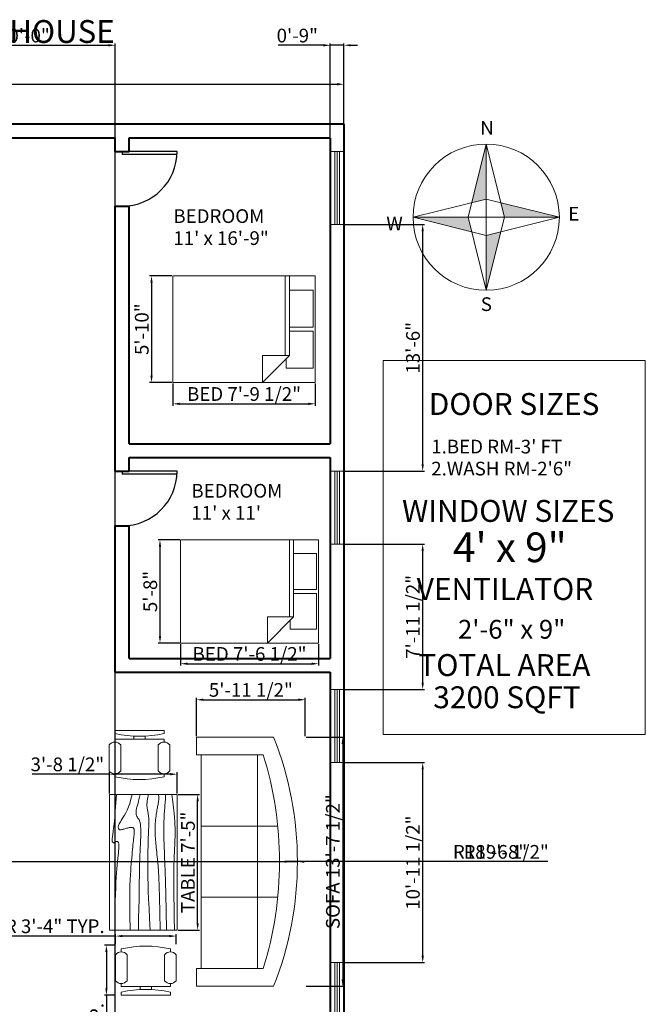
# Model space of a CAD drawing. Units: inches. Extents: x 2383 to 6214, y 970 to 3250.
# Tile 4 of 4: x 2721 to 3132, y 1500 to 2147. Entities that reach past the tile are written whole.
import ezdxf

# ---------------------------------------------------------------- set-up
doc = ezdxf.new("R2010")
doc.units = ezdxf.units.IN
for name, color, linetype, lineweight in [('A-ANNO-DIMS', 2, 'Continuous', 18), ('A-ANNO-LEGN', 7, 'Continuous', 18), ('A-ANNO-PATT', 7, 'Continuous', 13), ('A-ANNO-SYMB', 7, 'Continuous', 18), ('A-ANNO-TEXT', 7, 'Continuous', 18), ('A-AREA-IDEN', 7, 'Continuous', 18), ('A-DOOR', 4, 'Continuous', 25), ('A-FURN', 8, 'Continuous', 18), ('A-GLAZ', 4, 'Continuous', 18), ('A-WALL', 7, 'Continuous', 40)]:
    doc.layers.add(name, color=color, linetype=linetype, lineweight=lineweight)
doc.styles.get("Standard").update_dxf_attribs({"font": 'arial.ttf'})
doc.dimstyles.new('ISO-25', dxfattribs={"dimtxt": 9, "dimasz": 4.5, "dimexe": 1.25, "dimexo": 0.625, "dimtad": 1, "dimdec": 0, "dimlunit": 3, "dimtxsty": 'Standard', "dimcen": 2.5, "dimadec": 0, "dimazin": 0, "dimtfac": 1, "dimtdec": 0, "dimtmove": 0, "dimatfit": 3, "dimfxl": 1, "dimarcsym": 0})

# ---------------------------------------------------------------- blocks, each defined once
blk = doc.blocks.new('Sofa - Roundback 7 ft.')
for p, q in [((-12.00002, -32.4421), (-12.00003, -6.5971)), ((11.99997, -32.4421), (11.99998, -6.5971)), ((-36.000027, -34), (-36.000027, -11.4696)), ((35.99998, -34), (35.99998, -11.4696)), ((-35.999844, -13.3819), (35.9998, -13.3819)), ((-36.000027, -32.4421), (35.99998, -32.4421))]:
    blk.add_line(p, q)
for points in [[(-36.000027, -34), (-42.000027, -34), (-42.000027, -8)], [(41.99998, -8), (41.99998, -34), (35.99998, -34)]]:
    blk.add_lwpolyline(points)
for centre, radius, start, end in [((0, -114.25), 114.25, 68.43141, 111.5686), ((-0.00001, -127.1968), 121.1968, 72.72033, 107.2797)]:
    blk.add_arc(centre, radius, start, end)
blk = doc.blocks.new('Table - Rectangular Woodgrain 60 x 30 in.')
for p, q in [((0, 0), (0, -30)), ((60, 0), (0, 0)), ((60, -30), (60, 0)), ((0, -30), (60, -30))]:
    blk.add_line(p, q)
for points in [[(0, -2.4), (4.8155, -2.418), (9.0302, -2.4688), (12.709, -2.5477), (15.9167, -2.65), (18.7181, -2.7711), (21.1781, -2.9063), (23.3616, -3.0508), (25.3333, -3.2), (27.1477, -3.3495), (28.8172, -3.4958), (30.3437, -3.636), (31.7291, -3.7667), (32.9756, -3.8849), (34.0849, -3.9875), (35.059, -4.0714), (35.9, -4.1334), (36.6114, -4.1711), (37.2041, -4.1854), (37.6906, -4.1779), (38.0833, -4.15), (38.3948, -4.1034), (38.6375, -4.0396), (38.8239, -3.9602), (38.9666, -3.8667), (39.0764, -3.7608), (39.1573, -3.6448), (39.2116, -3.521), (39.2416, -3.3917), (39.2498, -3.2593), (39.2385, -3.1261), (39.21, -2.9944), (39.1666, -2.8667), (39.111, -2.7447), (39.0468, -2.6281), (38.978, -2.5163), (38.9083, -2.4083), (38.8418, -2.3035), (38.7823, -2.201), (38.7337, -2.1001), (38.7, -2), (38.6844, -1.9003), (38.6875, -1.8021), (38.7094, -1.707), (38.75, -1.6167), (38.8094, -1.5326), (38.8875, -1.4563), (38.9844, -1.3893), (39.1, -1.3333), (39.2351, -1.2896), (39.3937, -1.2583), (39.5804, -1.2396), (39.8, -1.2333), (40.057, -1.2396), (40.3562, -1.2583), (40.7023, -1.2896), (41.1, -1.3333), (41.5547, -1.3895), (42.0755, -1.4573), (42.6721, -1.5361), (43.3542, -1.625), (44.1316, -1.7233), (45.014, -1.8302), (46.0114, -1.9449), (47.1333, -2.0667), (48.3862, -2.1947), (49.7625, -2.3281), (51.2513, -2.4663), (52.8416, -2.6083), (54.5226, -2.7535), (56.2833, -2.9011), (58.1127, -3.0501), (60, -3.2)], [(0, -9.2), (6.5759, -9.0858), (11.9385, -9.0365), (16.2527, -9.0418), (19.6833, -9.0917), (22.3952, -9.1759), (24.5531, -9.2844), (26.322, -9.4069), (27.8666, -9.5333), (29.3241, -9.6553), (30.7203, -9.7719), (32.0532, -9.8837), (33.3208, -9.9917), (34.5213, -10.0965), (35.6526, -10.199), (36.7128, -10.2999), (37.7, -10.4), (38.6129, -10.4996), (39.4531, -10.5969), (40.223, -10.6895), (40.925, -10.775), (41.5613, -10.8512), (42.1344, -10.9156), (42.6465, -10.966), (43.1, -11), (43.4976, -11.0158), (43.8437, -11.0136), (44.143, -10.9942), (44.4, -10.9583), (44.6195, -10.9069), (44.8062, -10.8406), (44.9648, -10.7603), (45.1, -10.6667), (45.2155, -10.5598), (45.3114, -10.4365), (45.3871, -10.2929), (45.4416, -10.125), (45.4743, -9.929), (45.4844, -9.7011), (45.4709, -9.4371), (45.4333, -9.1333), (45.3716, -8.7883), (45.2896, -8.4104), (45.1919, -8.0107), (45.0833, -7.6), (44.9685, -7.1893), (44.8521, -6.7896), (44.7388, -6.4117), (44.6333, -6.0667), (44.54, -5.7628), (44.4614, -5.4979), (44.4001, -5.2675), (44.3583, -5.0667), (44.3384, -4.8909), (44.3427, -4.7354), (44.3736, -4.5956), (44.4333, -4.4667), (44.5236, -4.3453), (44.6427, -4.2333), (44.7884, -4.1339), (44.9583, -4.05), (45.1501, -3.9849), (45.3614, -3.9417), (45.59, -3.9234), (45.8333, -3.9333), (46.0915, -3.9749), (46.3734, -4.0531), (46.6906, -4.1736), (47.0542, -4.3417), (47.4756, -4.5629), (47.9661, -4.8427), (48.5372, -5.1866), (49.2, -5.6), (49.9676, -6.0844), (50.8594, -6.625), (51.8965, -7.2031), (53.1, -7.8), (54.491, -8.3969), (56.0906, -8.975), (57.9199, -9.5156), (60, -10)], [(0, -12.8), (5.1847, -12.9322), (9.6213, -13.0323), (13.3963, -13.1059), (16.5958, -13.1583), (19.3063, -13.1952), (21.614, -13.2219), (23.6054, -13.2439), (25.3666, -13.2667), (26.9728, -13.2947), (28.4531, -13.3281), (29.8256, -13.3663), (31.1083, -13.4083), (32.3191, -13.4535), (33.476, -13.501), (34.597, -13.5501), (35.7, -13.6), (36.7984, -13.6497), (37.8875, -13.6979), (38.9578, -13.743), (40, -13.7833), (41.0047, -13.8174), (41.9625, -13.8438), (42.864, -13.8607), (43.7, -13.8667), (44.4631, -13.8604), (45.1552, -13.8417), (45.7801, -13.8104), (46.3416, -13.7667), (46.8439, -13.7104), (47.2906, -13.6417), (47.6858, -13.5604), (48.0333, -13.4667), (48.3375, -13.3608), (48.6042, -13.2448), (48.8396, -13.121), (49.05, -12.9917), (49.2417, -12.8593), (49.4208, -12.7261), (49.5937, -12.5944), (49.7667, -12.4667), (49.9452, -12.3451), (50.1323, -12.2313), (50.3303, -12.1268), (50.5416, -12.0333), (50.7686, -11.9524), (51.0135, -11.8854), (51.2788, -11.8341), (51.5666, -11.8), (51.8785, -11.7843), (52.2116, -11.7865), (52.562, -11.8059), (52.926, -11.8417), (53.2998, -11.8931), (53.6795, -11.9594), (54.0614, -12.0397), (54.4416, -12.1333), (54.8223, -12.2401), (55.2293, -12.3625), (55.6942, -12.5037), (56.2489, -12.6667), (56.9251, -12.8547), (57.7545, -13.0708), (58.7689, -13.3182), (60, -13.6)], [(0, -18), (5.124, -17.7273), (9.6609, -17.5057), (13.6705, -17.3303), (17.2125, -17.1958), (20.3467, -17.0973), (23.1328, -17.0297), (25.6307, -16.9878), (27.9, -16.9667), (29.9928, -16.9617), (31.9302, -16.9703), (33.7254, -16.9907), (35.3917, -17.0208), (36.9423, -17.0588), (38.3906, -17.1026), (39.7499, -17.1503), (41.0333, -17.2), (42.2519, -17.2496), (43.4073, -17.2969), (44.4986, -17.3395), (45.525, -17.375), (46.4858, -17.4012), (47.3802, -17.4156), (48.2074, -17.416), (48.9667, -17.4), (49.6583, -17.3662), (50.2872, -17.3167), (50.8595, -17.2547), (51.3812, -17.1833), (51.8584, -17.1057), (52.2971, -17.025), (52.7034, -16.9443), (53.0833, -16.8667), (53.443, -16.7951), (53.789, -16.7313), (54.128, -16.6768), (54.4666, -16.6334), (54.8115, -16.6024), (55.1693, -16.5854), (55.5465, -16.5841), (55.95, -16.6), (56.3828, -16.6337), (56.8346, -16.6823), (57.2915, -16.7418), (57.7396, -16.8084), (58.165, -16.878), (58.5539, -16.9469), (58.8924, -17.0111), (59.1666, -17.0667), (59.3679, -17.1107), (59.5078, -17.1438), (59.6032, -17.1675), (59.6708, -17.1833), (59.7275, -17.193), (59.7901, -17.1979), (59.8753, -17.1998), (60, -17.2)], [(0, -22.4), (8.0098, -22.2501), (14.4094, -22.1011), (19.4168, -21.9535), (23.25, -21.8083), (26.1269, -21.6663), (28.2656, -21.5281), (29.884, -21.3947), (31.2, -21.2667), (32.3967, -21.1448), (33.5172, -21.0292), (34.5697, -20.9198), (35.5625, -20.8167), (36.5037, -20.7198), (37.4015, -20.6292), (38.2642, -20.5448), (39.1, -20.4667), (39.9164, -20.3951), (40.7187, -20.3313), (41.5117, -20.2768), (42.3, -20.2333), (43.0883, -20.2024), (43.8812, -20.1854), (44.6836, -20.1841), (45.5, -20.2), (46.3328, -20.234), (47.1747, -20.2844), (48.0163, -20.3488), (48.8479, -20.425), (49.66, -20.5106), (50.4429, -20.6031), (51.1872, -20.7004), (51.8833, -20.8), (52.5246, -20.8999), (53.1166, -20.9995), (53.6681, -21.0983), (54.1875, -21.1958), (54.6834, -21.2919), (55.1646, -21.3859), (55.6394, -21.4777), (56.1167, -21.5667), (56.6028, -21.6515), (57.0961, -21.7266), (57.5929, -21.7852), (58.0896, -21.8208), (58.5823, -21.8268), (59.0674, -21.7964), (59.5412, -21.723), (60, -21.6)], [(0, -25.2), (8.6355, -25.0504), (15.7026, -24.9031), (21.4049, -24.7606), (25.9458, -24.625), (29.529, -24.4988), (32.3578, -24.3844), (34.6359, -24.284), (36.5667, -24.2), (38.3213, -24.1341), (39.9417, -24.0854), (41.437, -24.0523), (42.8167, -24.0333), (44.0901, -24.0268), (45.2667, -24.0313), (46.3557, -24.0451), (47.3667, -24.0667), (48.309, -24.0947), (49.1928, -24.1287), (50.0284, -24.168), (50.826, -24.2125), (51.5959, -24.2617), (52.3483, -24.3151), (53.0935, -24.3725), (53.8417, -24.4334), (54.6009, -24.497), (55.3699, -24.561), (56.1454, -24.6226), (56.9239, -24.6792), (57.7021, -24.7279), (58.4764, -24.7662), (59.2435, -24.7911), (60, -24.8)], [(0, -28.8), (5.6867, -28.6681), (10.45, -28.5698), (14.407, -28.5012), (17.675, -28.4584), (20.3711, -28.4374), (22.6125, -28.4344), (24.5164, -28.4455), (26.2, -28.4667), (27.762, -28.4947), (29.2276, -28.5281), (30.6033, -28.5663), (31.8958, -28.6084), (33.1118, -28.6535), (34.2578, -28.7011), (35.3405, -28.7501), (36.3666, -28.8), (37.3443, -28.8497), (38.288, -28.8974), (39.2137, -28.9412), (40.1375, -28.9792), (41.0753, -29.0093), (42.0432, -29.0297), (43.0572, -29.0384), (44.1333, -29.0333), (45.2936, -29.0114), (46.5843, -28.9641), (48.0579, -28.8816), (49.7666, -28.7542), (51.7629, -28.5721), (54.0989, -28.3255), (56.8272, -28.0048), (60, -27.6)]]:
    blk.add_lwpolyline(points)
blk = doc.blocks.new('Chair - Desk')
for p, q in [((-8.5, 0), (-8.5, -1)), ((-8.5, 0), (8.5, 0)), ((8.5, 0), (8.5, -1)), ((-8.5, -3), (-8.5, -4)), ((-8.5, -3), (8.5, -3)), ((-2, -3), (-2, -1.9355)), ((2, -1.9576), (2, -3)), ((8.5, -3), (8.5, -4)), ((-10.5, -5), (-10.5, -14)), ((-6.5, -14), (-6.5, -5)), ((6.5, -5), (6.5, -14)), ((10.5, -14), (10.5, -5)), ((-8.5, -15), (-8.5, -16)), ((8.5, -15), (8.5, -16))]:
    blk.add_line(p, q)
for centre, radius, start, end in [((0, 34.625), 36.625, 256.5803, 283.4197), ((-8.5, -6.5), 2.5, 36.8699, 143.1301), ((8.5, -6.5), 2.5, 36.8699, 143.1301), ((-8.5, -12.5), 2.5, 216.8699, 323.1301), ((0, 19.625), 36.625, 256.5803, 283.4197), ((8.5, -12.5), 2.5, 216.8699, 323.1301)]:
    blk.add_arc(centre, radius, start, end)
blk = doc.blocks.new('Bed - Queen')
for p, q in [((0, -80.00003), (0, 0)), ((0, 0), (59.99999, 0)), ((59.99999, 0), (59.99999, -80.00003)), ((7.99999, -1.2), (28.79998, -1.2)), ((7.99999, -14.4), (7.99999, -1.2)), ((28.79998, -1.2), (28.79998, -14.4)), ((31.19999, -1.2), (51.99999, -1.2)), ((31.19999, -14.4), (31.19999, -1.2)), ((51.99999, -1.2), (51.99999, -16.4)), ((0, -14.4), (44.8, -14.4)), ((59.99999, -29.6), (44.8, -14.4)), ((44.8, -14.4), (44.8, -29.6)), ((51.99999, -16.4), (46.79936, -16.4)), ((44.8, -16.8), (0, -16.8)), ((44.8, -29.6), (59.99999, -29.6)), ((59.99999, -80.00003), (0, -80.00003))]:
    blk.add_line(p, q)
blk = doc.blocks.new('*D14')
at = {"layer": 'A-ANNO-DIMS', "color": 0, "lineweight": -2, "transparency": 16777216}
for p, q in [((2453.83, 2079.3), (2453.83, 2106.04)), ((2458.33, 2104.79), (2929.33, 2104.79)), ((2933.83, 2079.3), (2933.83, 2106.04))]:
    blk.add_line(p, q, dxfattribs=at)
at = {"layer": 'A-ANNO-DIMS', "color": 0, "transparency": 16777216}
for points in [[(2458.33, 2105.54), (2458.33, 2104.04), (2453.83, 2104.79)], [(2929.33, 2105.54), (2929.33, 2104.04), (2933.83, 2104.79)]]:
    blk.add_solid(points, dxfattribs=at)
at = {"layer": 'Defpoints', "color": 0, "transparency": 16777216}
for p in [(2933.83, 2104.79), (2453.83, 2078.68), (2933.83, 2078.68)]:
    blk.add_point(p, dxfattribs=at)
at = {"layer": 'A-ANNO-DIMS', "color": 0, "transparency": 16777216, "insert": (2693.83, 2110.01), "char_height": 9, "attachment_point": 5}
blk.add_mtext("40'", dxfattribs=at)
blk = doc.blocks.new('*U17')
for q in [(-11.92, -24), (11.92, -24)]:
    blk.add_line((0, 24), q)
blk = doc.blocks.new('*U18')
at = {"layer": 'A-ANNO-SYMB', "color": 0, "linetype": 'ByBlock', "lineweight": -2, "transparency": 16777216}
blk.add_blockref('*U17', (3112.93, 1965.9), dxfattribs=at)
for p, rotation in [((3088.93, 1941.9), 90), ((3136.93, 1941.9), 270), ((3112.93, 1917.9), 180)]:
    blk.add_blockref('*U17', p, dxfattribs=dict(at, rotation=rotation))
blk = doc.blocks.new('DOOR-SWING-36IN')
for p, q in [((36, 36), (0, 36)), ((0, 36), (0, 34)), ((36, 34), (0, 34))]:
    blk.add_line(p, q)
blk.add_arc((0, 36), 36, 270, 0)
blk = doc.blocks.new('WINDOW-48X9IN')
for p, q in [((3, 0), (3, 48)), ((4.5, 0), (4.5, 48)), ((6, 0), (6, 48))]:
    blk.add_line(p, q)
blk.add_lwpolyline([(0, 0), (0, 48), (9, 48), (9, 0)], close=True)
blk = doc.blocks.new('*D25')
at = {"layer": 'A-ANNO-DIMS', "color": 0, "lineweight": -2, "transparency": 16777216}
for p, q in [((2821.58, 1908.27), (2821.58, 1893.63)), ((2914.97, 1908.27), (2914.97, 1893.63)), ((2826.08, 1894.88), (2910.47, 1894.88))]:
    blk.add_line(p, q, dxfattribs=at)
at = {"layer": 'A-ANNO-DIMS', "color": 0, "transparency": 16777216}
for points in [[(2826.08, 1895.63), (2826.08, 1894.13), (2821.58, 1894.88)], [(2910.47, 1895.63), (2910.47, 1894.13), (2914.97, 1894.88)]]:
    blk.add_solid(points, dxfattribs=at)
at = {"layer": 'Defpoints', "color": 0, "transparency": 16777216}
for p in [(2821.58, 1908.89), (2914.97, 1908.89), (2914.97, 1894.88)]:
    blk.add_point(p, dxfattribs=at)
at = {"layer": 'A-ANNO-DIMS', "color": 0, "transparency": 16777216, "insert": (2868.27, 1900.16), "char_height": 9, "attachment_point": 5}
blk.add_mtext('BED 7\'-9 1/2"', dxfattribs=at)
blk = doc.blocks.new('*D26')
at = {"layer": 'A-ANNO-DIMS', "color": 0, "lineweight": -2, "transparency": 16777216}
for p, q in [((2820.95, 1978.94), (2806.32, 1978.94)), ((2807.57, 1974.44), (2807.57, 1913.39)), ((2820.95, 1908.89), (2806.32, 1908.89))]:
    blk.add_line(p, q, dxfattribs=at)
at = {"layer": 'A-ANNO-DIMS', "color": 0, "transparency": 16777216}
for points in [[(2806.82, 1974.44), (2808.32, 1974.44), (2807.57, 1978.94)], [(2806.82, 1913.39), (2808.32, 1913.39), (2807.57, 1908.89)]]:
    blk.add_solid(points, dxfattribs=at)
at = {"layer": 'Defpoints', "color": 0, "transparency": 16777216}
for p in [(2821.58, 1978.94), (2807.57, 1908.89), (2821.58, 1908.89)]:
    blk.add_point(p, dxfattribs=at)
at = {"layer": 'A-ANNO-DIMS', "color": 0, "transparency": 16777216, "insert": (2802.35, 1943.91), "char_height": 9, "attachment_point": 5, "rotation": 90}
blk.add_mtext('5\'-10"', dxfattribs=at)
blk = doc.blocks.new('*D27')
at = {"layer": 'A-ANNO-DIMS', "color": 0, "lineweight": -2, "transparency": 16777216}
for p, q in [((2826.7, 1737.11), (2826.7, 1722.92)), ((2917.12, 1737.11), (2917.12, 1722.92)), ((2831.2, 1724.17), (2912.62, 1724.17))]:
    blk.add_line(p, q, dxfattribs=at)
at = {"layer": 'A-ANNO-DIMS', "color": 0, "transparency": 16777216}
for points in [[(2831.2, 1724.92), (2831.2, 1723.42), (2826.7, 1724.17)], [(2912.62, 1724.92), (2912.62, 1723.42), (2917.12, 1724.17)]]:
    blk.add_solid(points, dxfattribs=at)
at = {"layer": 'Defpoints', "color": 0, "transparency": 16777216}
for p in [(2826.7, 1737.73), (2917.12, 1737.73), (2917.12, 1724.17)]:
    blk.add_point(p, dxfattribs=at)
at = {"layer": 'A-ANNO-DIMS', "color": 0, "transparency": 16777216, "insert": (2871.91, 1729.45), "char_height": 9, "attachment_point": 5}
blk.add_mtext('BED 7\'-6 1/2"', dxfattribs=at)
blk = doc.blocks.new('*D28')
at = {"layer": 'A-ANNO-DIMS', "color": 0, "lineweight": -2, "transparency": 16777216}
for p, q in [((2826.07, 1805.55), (2811.89, 1805.55)), ((2813.14, 1801.05), (2813.14, 1742.23)), ((2826.07, 1737.73), (2811.89, 1737.73))]:
    blk.add_line(p, q, dxfattribs=at)
at = {"layer": 'A-ANNO-DIMS', "color": 0, "transparency": 16777216}
for points in [[(2812.39, 1801.05), (2813.89, 1801.05), (2813.14, 1805.55)], [(2812.39, 1742.23), (2813.89, 1742.23), (2813.14, 1737.73)]]:
    blk.add_solid(points, dxfattribs=at)
at = {"layer": 'Defpoints', "color": 0, "transparency": 16777216}
for p in [(2826.7, 1805.55), (2813.14, 1737.73), (2826.7, 1737.73)]:
    blk.add_point(p, dxfattribs=at)
at = {"layer": 'A-ANNO-DIMS', "color": 0, "transparency": 16777216, "insert": (2807.92, 1771.64), "char_height": 9, "attachment_point": 5, "rotation": 90}
blk.add_mtext('5\'-8"', dxfattribs=at)
blk = doc.blocks.new('*D37')
at = {"layer": 'A-ANNO-DIMS', "color": 0, "lineweight": -2, "transparency": 16777216}
for p, q in [((2783.96, 1539.97), (2783.96, 1546.56)), ((2823.73, 1539.97), (2823.73, 1546.56)), ((2783.96, 1545.31), (2680.84, 1545.31)), ((2819.23, 1545.31), (2788.46, 1545.31))]:
    blk.add_line(p, q, dxfattribs=at)
at = {"layer": 'A-ANNO-DIMS', "color": 0, "transparency": 16777216}
for points in [[(2788.46, 1546.06), (2788.46, 1544.56), (2783.96, 1545.31)], [(2819.23, 1546.06), (2819.23, 1544.56), (2823.73, 1545.31)]]:
    blk.add_solid(points, dxfattribs=at)
at = {"layer": 'Defpoints', "color": 0, "transparency": 16777216}
for p in [(2783.96, 1545.31), (2783.96, 1539.35), (2823.73, 1539.35)]:
    blk.add_point(p, dxfattribs=at)
at = {"layer": 'A-ANNO-DIMS', "color": 0, "transparency": 16777216, "insert": (2730.15, 1550.6), "char_height": 9, "attachment_point": 5}
blk.add_mtext('CHAIR 3\'-4" TYP.', dxfattribs=at)
blk = doc.blocks.new('*D38')
at = {"layer": 'A-ANNO-DIMS', "color": 0, "lineweight": -2, "transparency": 16777216}
for p, q in [((2783.33, 1539.35), (2776.74, 1539.35)), ((2777.99, 1534.85), (2777.99, 1511.02)), ((2783.33, 1506.52), (2776.74, 1506.52)), ((2777.99, 1506.52), (2777.99, 1445.76))]:
    blk.add_line(p, q, dxfattribs=at)
at = {"layer": 'A-ANNO-DIMS', "color": 0, "transparency": 16777216}
for points in [[(2777.24, 1534.85), (2778.74, 1534.85), (2777.99, 1539.35)], [(2777.24, 1511.02), (2778.74, 1511.02), (2777.99, 1506.52)]]:
    blk.add_solid(points, dxfattribs=at)
at = {"layer": 'Defpoints', "color": 0, "transparency": 16777216}
for p in [(2783.96, 1539.35), (2777.99, 1506.52), (2783.96, 1506.52)]:
    blk.add_point(p, dxfattribs=at)
at = {"layer": 'A-ANNO-DIMS', "color": 0, "transparency": 16777216, "insert": (2772.77, 1473.89), "char_height": 9, "attachment_point": 5, "rotation": 90}
blk.add_mtext('2\'-9" TYP.', dxfattribs=at)
blk = doc.blocks.new('*D41')
at = {"layer": 'A-ANNO-DIMS', "color": 0, "lineweight": -2, "transparency": 16777216}
for p, q in [((2909.11, 1675.99), (2934.27, 1675.99)), ((2933.02, 1671.49), (2933.02, 1516.87)), ((2909.11, 1512.37), (2934.27, 1512.37))]:
    blk.add_line(p, q, dxfattribs=at)
at = {"layer": 'A-ANNO-DIMS', "color": 0, "transparency": 16777216}
for points in [[(2932.27, 1671.49), (2933.77, 1671.49), (2933.02, 1675.99)], [(2932.27, 1516.87), (2933.77, 1516.87), (2933.02, 1512.37)]]:
    blk.add_solid(points, dxfattribs=at)
at = {"layer": 'Defpoints', "color": 0, "transparency": 16777216}
for p in [(2908.48, 1675.99), (2908.48, 1512.37), (2933.02, 1512.37)]:
    blk.add_point(p, dxfattribs=at)
at = {"layer": 'A-ANNO-DIMS', "color": 0, "transparency": 16777216, "insert": (2927.74, 1594.18), "char_height": 9, "attachment_point": 5, "rotation": 90}
blk.add_mtext('SOFA 13\'-7 1/2"', dxfattribs=at)
blk = doc.blocks.new('*D42')
at = {"layer": 'A-ANNO-DIMS', "color": 0, "lineweight": -2, "transparency": 16777216}
for p, q in [((2837.06, 1676.61), (2837.06, 1701.78)), ((2908.48, 1676.61), (2908.48, 1701.78)), ((2841.56, 1700.53), (2903.98, 1700.53))]:
    blk.add_line(p, q, dxfattribs=at)
at = {"layer": 'A-ANNO-DIMS', "color": 0, "transparency": 16777216}
for points in [[(2841.56, 1701.28), (2841.56, 1699.78), (2837.06, 1700.53)], [(2903.98, 1701.28), (2903.98, 1699.78), (2908.48, 1700.53)]]:
    blk.add_solid(points, dxfattribs=at)
at = {"layer": 'Defpoints', "color": 0, "transparency": 16777216}
for p in [(2908.48, 1700.53), (2837.06, 1675.99), (2908.48, 1675.99)]:
    blk.add_point(p, dxfattribs=at)
at = {"layer": 'A-ANNO-DIMS', "color": 0, "transparency": 16777216, "insert": (2872.77, 1705.81), "char_height": 9, "attachment_point": 5}
blk.add_mtext('5\'-11 1/2"', dxfattribs=at)
blk = doc.blocks.new('*D45')
at = {"layer": 'A-ANNO-DIMS', "color": 0, "lineweight": -2, "transparency": 16777216}
for p, q in [((2825.11, 1638.27), (2839.1, 1638.27)), ((2837.85, 1553.68), (2837.85, 1633.77)), ((2825.11, 1549.18), (2839.1, 1549.18))]:
    blk.add_line(p, q, dxfattribs=at)
at = {"layer": 'A-ANNO-DIMS', "color": 0, "transparency": 16777216}
for points in [[(2837.1, 1633.77), (2838.6, 1633.77), (2837.85, 1638.27)], [(2837.1, 1553.68), (2838.6, 1553.68), (2837.85, 1549.18)]]:
    blk.add_solid(points, dxfattribs=at)
at = {"layer": 'Defpoints', "color": 0, "transparency": 16777216}
for p in [(2824.48, 1638.27), (2837.85, 1638.27), (2824.48, 1549.18)]:
    blk.add_point(p, dxfattribs=at)
at = {"layer": 'A-ANNO-DIMS', "color": 0, "transparency": 16777216, "insert": (2832.65, 1593.72), "char_height": 9, "attachment_point": 5, "rotation": 90}
blk.add_mtext('TABLE 7\'-5"', dxfattribs=at)
blk = doc.blocks.new('*D46')
at = {"layer": 'A-ANNO-DIMS', "color": 0, "lineweight": -2, "transparency": 16777216}
for p, q in [((2779.94, 1651.63), (2729.3, 1651.63)), ((2779.94, 1638.9), (2779.94, 1652.88)), ((2819.98, 1651.63), (2784.44, 1651.63)), ((2824.48, 1638.9), (2824.48, 1652.88))]:
    blk.add_line(p, q, dxfattribs=at)
at = {"layer": 'A-ANNO-DIMS', "color": 0, "transparency": 16777216}
for points in [[(2784.44, 1652.38), (2784.44, 1650.88), (2779.94, 1651.63)], [(2819.98, 1652.38), (2819.98, 1650.88), (2824.48, 1651.63)]]:
    blk.add_solid(points, dxfattribs=at)
at = {"layer": 'Defpoints', "color": 0, "transparency": 16777216}
for p in [(2779.94, 1651.63), (2779.94, 1638.27), (2824.48, 1638.27)]:
    blk.add_point(p, dxfattribs=at)
at = {"layer": 'A-ANNO-DIMS', "color": 0, "transparency": 16777216, "insert": (2752.37, 1656.92), "char_height": 9, "attachment_point": 5}
blk.add_mtext('3\'-8 1/2"', dxfattribs=at)
blk = doc.blocks.new('*D56')
at = {"layer": 'A-ANNO-DIMS', "color": 0, "lineweight": -2, "transparency": 16777216}
for p, q in [((2663.83, 1128.3), (2663.83, 2131.63)), ((2668.33, 2130.38), (2779.33, 2130.38)), ((2783.83, 1128.3), (2783.83, 2131.63))]:
    blk.add_line(p, q, dxfattribs=at)
at = {"layer": 'A-ANNO-DIMS', "color": 0, "transparency": 16777216}
for points in [[(2668.33, 2131.13), (2668.33, 2129.63), (2663.83, 2130.38)], [(2779.33, 2131.13), (2779.33, 2129.63), (2783.83, 2130.38)]]:
    blk.add_solid(points, dxfattribs=at)
at = {"layer": 'Defpoints', "color": 0, "transparency": 16777216}
for p in [(2783.83, 2130.38), (2663.83, 1127.68), (2783.83, 1127.68)]:
    blk.add_point(p, dxfattribs=at)
at = {"layer": 'A-ANNO-DIMS', "color": 0, "transparency": 16777216, "insert": (2723.83, 2135.6), "char_height": 9, "attachment_point": 5}
blk.add_mtext('10\'-0"', dxfattribs=at)
blk = doc.blocks.new('*D58')
at = {"layer": 'A-ANNO-DIMS', "color": 0, "lineweight": -2, "transparency": 16777216}
for p, q in [((2920.33, 2130.38), (2890.65, 2130.38)), ((2924.83, 2070.3), (2924.83, 2131.63)), ((2933.83, 2130.38), (2924.83, 2130.38)), ((2933.83, 2079.3), (2933.83, 2131.63)), ((2938.33, 2130.38), (2942.83, 2130.38))]:
    blk.add_line(p, q, dxfattribs=at)
at = {"layer": 'A-ANNO-DIMS', "color": 0, "transparency": 16777216}
for points in [[(2920.33, 2131.13), (2920.33, 2129.63), (2924.83, 2130.38)], [(2938.33, 2131.13), (2938.33, 2129.63), (2933.83, 2130.38)]]:
    blk.add_solid(points, dxfattribs=at)
at = {"layer": 'Defpoints', "color": 0, "transparency": 16777216}
for p in [(2924.83, 2130.38), (2933.83, 2078.68), (2924.83, 2069.68)]:
    blk.add_point(p, dxfattribs=at)
at = {"layer": 'A-ANNO-DIMS', "color": 0, "transparency": 16777216, "insert": (2903.24, 2135.6), "char_height": 9, "attachment_point": 5}
blk.add_mtext('0\'-9"', dxfattribs=at)
blk = doc.blocks.new('*D68')
at = {"layer": 'A-ANNO-DIMS', "color": 0, "lineweight": -2, "transparency": 16777216}
for p, q in [((2934.45, 1659.23), (2986.78, 1659.23)), ((2985.53, 1532.35), (2985.53, 1654.73)), ((2934.45, 1527.85), (2986.78, 1527.85))]:
    blk.add_line(p, q, dxfattribs=at)
at = {"layer": 'A-ANNO-DIMS', "color": 0, "transparency": 16777216}
for points in [[(2984.78, 1654.73), (2986.28, 1654.73), (2985.53, 1659.23)], [(2984.78, 1532.35), (2986.28, 1532.35), (2985.53, 1527.85)]]:
    blk.add_solid(points, dxfattribs=at)
at = {"layer": 'Defpoints', "color": 0, "transparency": 16777216}
for p in [(2933.83, 1659.23), (2985.53, 1659.23), (2933.83, 1527.85)]:
    blk.add_point(p, dxfattribs=at)
at = {"layer": 'A-ANNO-DIMS', "color": 0, "transparency": 16777216, "insert": (2980.25, 1593.54), "char_height": 9, "attachment_point": 5, "rotation": 90}
blk.add_mtext('10\'-11 1/2"', dxfattribs=at)
blk = doc.blocks.new('*D69')
at = {"layer": 'A-ANNO-DIMS', "color": 0, "lineweight": -2, "transparency": 16777216}
for p, q in [((2934.45, 1802.68), (2986.78, 1802.68)), ((2985.53, 1711.73), (2985.53, 1798.18)), ((2934.45, 1707.23), (2986.78, 1707.23))]:
    blk.add_line(p, q, dxfattribs=at)
at = {"layer": 'A-ANNO-DIMS', "color": 0, "transparency": 16777216}
for points in [[(2984.78, 1798.18), (2986.28, 1798.18), (2985.53, 1802.68)], [(2984.78, 1711.73), (2986.28, 1711.73), (2985.53, 1707.23)]]:
    blk.add_solid(points, dxfattribs=at)
at = {"layer": 'Defpoints', "color": 0, "transparency": 16777216}
for p in [(2933.83, 1802.68), (2985.53, 1802.68), (2933.83, 1707.23)]:
    blk.add_point(p, dxfattribs=at)
at = {"layer": 'A-ANNO-DIMS', "color": 0, "transparency": 16777216, "insert": (2980.25, 1754.95), "char_height": 9, "attachment_point": 5, "rotation": 90}
blk.add_mtext('7\'-11 1/2"', dxfattribs=at)
blk = doc.blocks.new('*D70')
at = {"layer": 'A-ANNO-DIMS', "color": 0, "lineweight": -2, "transparency": 16777216}
for p, q in [((2934.45, 2012.68), (2986.78, 2012.68)), ((2985.53, 1855.18), (2985.53, 2008.18)), ((2934.45, 1850.68), (2986.78, 1850.68))]:
    blk.add_line(p, q, dxfattribs=at)
at = {"layer": 'A-ANNO-DIMS', "color": 0, "transparency": 16777216}
for points in [[(2984.78, 2008.18), (2986.28, 2008.18), (2985.53, 2012.68)], [(2984.78, 1855.18), (2986.28, 1855.18), (2985.53, 1850.68)]]:
    blk.add_solid(points, dxfattribs=at)
at = {"layer": 'Defpoints', "color": 0, "transparency": 16777216}
for p in [(2933.83, 2012.68), (2985.53, 2012.68), (2933.83, 1850.68)]:
    blk.add_point(p, dxfattribs=at)
at = {"layer": 'A-ANNO-DIMS', "color": 0, "transparency": 16777216, "insert": (2980.3, 1931.68), "char_height": 9, "attachment_point": 5, "rotation": 90}
blk.add_mtext('13\'-6"', dxfattribs=at)
blk = doc.blocks.new('*D71')
at = {"layer": 'A-ANNO-DIMS', "color": 0, "lineweight": -2, "transparency": 16777216}
for p, q in [((2655.53, 1594.18), (2891.6, 1594.18)), ((3053.63, 1594.18), (2896.1, 1594.18))]:
    blk.add_line(p, q, dxfattribs=at)
at = {"layer": 'A-ANNO-DIMS', "color": 0, "transparency": 16777216}
blk.add_solid([(2896.1, 1594.93), (2896.1, 1593.43), (2891.6, 1594.18)], dxfattribs=at)
at = {"layer": 'Defpoints', "color": 0, "transparency": 16777216}
for p in [(2655.53, 1594.18), (2891.6, 1594.18)]:
    blk.add_point(p, dxfattribs=at)
at = {"layer": 'A-ANNO-DIMS', "color": 0, "transparency": 16777216, "insert": (3033.24, 1599.4), "char_height": 9, "attachment_point": 5, "rotation": 0.00005}
blk.add_mtext('R19\'-8"', dxfattribs=at)
blk = doc.blocks.new('*D72')
at = {"layer": 'A-ANNO-DIMS', "color": 0, "lineweight": -2, "transparency": 16777216}
for p, q in [((2680.75, 1594.18), (2903.29, 1594.18)), ((3067.69, 1594.18), (2907.79, 1594.18))]:
    blk.add_line(p, q, dxfattribs=at)
at = {"layer": 'A-ANNO-DIMS', "color": 0, "transparency": 16777216}
blk.add_solid([(2907.79, 1594.93), (2907.79, 1593.43), (2903.29, 1594.18)], dxfattribs=at)
at = {"layer": 'Defpoints', "color": 0, "transparency": 16777216}
for p in [(2680.75, 1594.18), (2903.29, 1594.18)]:
    blk.add_point(p, dxfattribs=at)
at = {"layer": 'A-ANNO-DIMS', "color": 0, "transparency": 16777216, "insert": (3036.81, 1599.46), "char_height": 9, "attachment_point": 5, "rotation": 0.00005}
blk.add_mtext('R18\'-6 1/2"', dxfattribs=at)

msp = doc.modelspace()

# ---------------------------------------------------------------- hatches: boundary and pattern name
at = {"layer": 'A-ANNO-PATT'}
h = msp.add_hatch(color=256, dxfattribs=at)
h.dxf.hatch_style = 1
h.paths.add_polyline_path([(3027.19, 2065.45), (3017.64, 2026.99), (3027.19, 2029.37)])
h.paths.add_polyline_path([(3015.27, 2017.45), (2979.19, 2017.45), (3017.64, 2007.9)])
h.paths.add_polyline_path([(3027.19, 1969.45), (3036.74, 2007.9), (3027.19, 2005.52)])
h.paths.add_polyline_path([(3075.19, 2017.45), (3036.74, 2026.99), (3039.11, 2017.45)])

# ---------------------------------------------------------------- linework, layer by layer
at = {"layer": 'A-ANNO-LEGN'}
for p, q in [((2959.6, 1923.33), (2959.6, 1726.26)), ((2959.6, 1923.33), (3131.59, 1923.33)), ((3131.59, 1724.57), (3131.59, 1923.33)), ((2959.6, 1726.26), (2959.6, 1726.26)), ((2959.6, 1726.26), (2959.6, 1677.63)), ((3131.59, 1677.63), (3131.59, 1724.57)), ((2959.6, 1677.63), (3131.59, 1677.63))]:
    msp.add_line(p, q, dxfattribs=at)
at = {"layer": 'A-ANNO-SYMB'}
for p, q in [((3027.19, 2065.45), (3027.19, 1969.45)), ((2979.19, 2017.45), (3075.19, 2017.45))]:
    msp.add_line(p, q, dxfattribs=at)
msp.add_circle((3027.19, 2017.45), 48, dxfattribs=at)
at = {"layer": 'A-WALL'}
for p, q in [((2453.83, 2078.68), (2933.83, 2078.68)), ((2933.83, 2078.68), (2933.83, 1118.68)), ((2663.83, 2069.68), (2783.83, 2069.68)), ((2783.83, 2060.68), (2783.83, 2069.68)), ((2792.83, 2060.68), (2792.83, 2069.68)), ((2792.83, 2069.68), (2924.83, 2069.68)), ((2924.83, 2069.68), (2924.83, 1868.68)), ((2783.83, 2060.68), (2792.83, 2060.68)), ((2783.83, 2024.68), (2792.83, 2024.68)), ((2783.83, 1850.68), (2783.83, 2024.68)), ((2792.83, 1868.68), (2792.83, 2024.68)), ((2792.83, 1868.68), (2924.83, 1868.68)), ((2792.83, 1859.68), (2924.83, 1859.68)), ((2792.83, 1850.68), (2792.83, 1859.68)), ((2924.83, 1859.68), (2924.83, 1727.68)), ((2783.83, 1850.68), (2792.83, 1850.68)), ((2783.83, 1718.68), (2783.83, 1814.68)), ((2783.83, 1814.68), (2792.83, 1814.68)), ((2792.83, 1727.68), (2792.83, 1814.68)), ((2792.83, 1727.68), (2924.83, 1727.68)), ((2783.83, 1718.68), (2924.83, 1718.68)), ((2924.83, 1718.68), (2924.83, 1469.68))]:
    msp.add_line(p, q, dxfattribs=at)

# ---------------------------------------------------------------- block references
at = {"layer": 'A-ANNO-SYMB'}
msp.add_blockref('*U18', (-85.74, 75.54), dxfattribs=at)
at = {"layer": 'A-DOOR'}
for p in [(2788.33, 2024.68), (2788.33, 1814.68)]:
    msp.add_blockref('DOOR-SWING-36IN', p, dxfattribs=at)
at = {"layer": 'A-FURN'}
for name, p, xscale, yscale, zscale, rotation in [('Bed - Queen', (2914.97, 1978.94), 1.167372111064088, 1.167372111064088, 1.167372111064088, 270), ('Bed - Queen', (2917.12, 1805.55), 1.130251999547992, 1.130251999547992, 1.130251999547992, 270), ('Sofa - Roundback 7 ft.', (2903.29, 1594.18), 1.947830468078298, 1.947830468078298, 1.947830468078298, 270), ('Table - Rectangular Woodgrain 60 x 30 in.', (2779.94, 1549.18), 1.484872478447348, 1.484872478447348, 1.484872478447348, 90), ('Chair - Desk', (2803.84, 1506.52), 1.893945549891067, 1.893945549891067, 1.893945549891067, 180)]:
    msp.add_blockref(name, p, dxfattribs=dict(at, xscale=xscale, yscale=yscale, zscale=zscale, rotation=rotation))
at = {"layer": 'A-FURN', "xscale": 1.893945549891067, "yscale": 1.893945549891067, "zscale": 1.893945549891067}
msp.add_blockref('Chair - Desk', (2799.67, 1680.3), dxfattribs=at)
at = {"layer": 'A-GLAZ'}
for p in [(2924.83, 2012.68), (2924.83, 1802.68), (2924.83, 1659.23), (2924.83, 1479.85)]:
    msp.add_blockref('WINDOW-48X9IN', p, dxfattribs=at)

# ---------------------------------------------------------------- texts
at = {"layer": 'A-ANNO-SYMB'}
for s, p in [('N ', (3023.3, 2071.59)), ('E', (3081.04, 2015.26)), ('W', (2961.64, 2008.81)), ('S', (3023.64, 1955.84))]:
    msp.add_text(s, height=9, dxfattribs=at).set_placement(p)
at = {"layer": 'A-ANNO-TEXT'}
for s, height, p in [('SOUTH FACING HOUSE', 15, (2564.12, 2131.92)), ('DOOR SIZES', 14.38, (2989.51, 1887.57)), ("1.BED RM-3' FT", 9, (2991.14, 1862.3)), ('2.WASH RM-2\'6"', 9, (2991.14, 1847.84)), ('WINDOW SIZES', 14.3801, (2971.98, 1817.35)), ('4\' x 9"', 19.499, (3005.39, 1790.89)), ('VENTILATOR', 14.38, (2981.59, 1766.05)), ('2\'-6" x 9"', 12.334, (3008.71, 1740.65)), ('TOTAL AREA ', 14.3801, (2982.68, 1716.12)), ('3200 SQFT', 14.38, (2992.46, 1694.96))]:
    msp.add_text(s, height=height, dxfattribs=at).set_placement(p)
at = {"layer": 'A-AREA-IDEN'}
for s, p in [('BEDROOM', (2821.9, 2013.68)), ('11\' x 16\'-9"', (2821.9, 1999.22)), ('BEDROOM', (2833.72, 1833.27)), ("11' x 11'", (2833.72, 1818.81))]:
    msp.add_text(s, height=9, dxfattribs=at).set_placement(p)

# ---------------------------------------------------------------- dimensions: what is measured, and where the dimension line sits
at = {"layer": 'A-ANNO-DIMS'}
for base, p1, p2, override, picture, middle in [((2783.83, 2130.38), (2663.83, 1127.68), (2783.83, 1127.68), {"dimdec": 1, "dimlfac": 1, "dimrnd": 0, "dimzin": 1, "dimdsep": 46, "dimlunit": 4, "dimfrac": 2}, '*D56', (2723.83, 2135.6)), ((2924.83, 2130.38), (2933.83, 2078.68), (2924.83, 2069.68), {"dimdec": 1, "dimlfac": 1, "dimrnd": 0, "dimzin": 1, "dimdsep": 46, "dimlunit": 4, "dimfrac": 2}, '*D58', (2903.24, 2135.6)), ((2933.83, 2104.79), (2453.83, 2078.68), (2933.83, 2078.68), {"dimclrd": 0, "dimclre": 0, "dimclrt": 0}, '*D14', (2693.83, 2110.01)), ((2908.48, 1700.53), (2837.06, 1675.99), (2908.48, 1675.99), {"dimdec": 1, "dimlfac": 1, "dimrnd": 0, "dimzin": 1, "dimdsep": 46, "dimlunit": 4, "dimfrac": 2}, '*D42', (2872.77, 1705.81))]:
    dim = msp.add_linear_dim(base=base, p1=p1, p2=p2, dimstyle='ISO-25', override=override, dxfattribs=at)
    dim.commit()
    dim.dimension.update_dxf_attribs({"geometry": picture, "text_midpoint": middle})
for base, p1, p2, angle, picture, middle in [((2985.53, 2012.68), (2933.83, 1850.68), (2933.83, 2012.68), 90, '*D70', (2980.3, 1931.68)), ((2807.5693, 1908.8933), (2821.5778, 1978.9356), (2821.5778, 1908.8933), 270, '*D26', (2802.3491, 1943.9145)), ((2813.14, 1737.73), (2826.7, 1805.55), (2826.7, 1737.73), 270, '*D28', (2807.92, 1771.64)), ((2985.5281, 1802.6798), (2933.8281, 1707.2296), (2933.8281, 1802.6798), 90, '*D69', (2980.2496, 1754.9547)), ((2779.94, 1651.63), (2824.48, 1638.27), (2779.94, 1638.27), 180, '*D46', (2752.37, 1656.92)), ((2985.53, 1659.23), (2933.83, 1527.85), (2933.83, 1659.23), 90, '*D68', (2980.25, 1593.54))]:
    dim = msp.add_linear_dim(base=base, p1=p1, p2=p2, angle=angle, dimstyle='ISO-25', override={"dimdec": 1, "dimlfac": 1, "dimrnd": 0, "dimzin": 1, "dimdsep": 46, "dimlunit": 4, "dimfrac": 2}, dxfattribs=at)
    dim.commit()
    dim.dimension.update_dxf_attribs({"geometry": picture, "text_midpoint": middle})
for base, p1, p2, picture, middle in [((2914.97, 1894.88), (2821.58, 1908.89), (2914.97, 1908.89), '*D25', (2868.27, 1900.16)), ((2917.12, 1724.17), (2826.7, 1737.73), (2917.12, 1737.73), '*D27', (2871.91, 1729.45))]:
    dim = msp.add_linear_dim(base=base, p1=p1, p2=p2, text='BED <>', dimstyle='ISO-25', override={"dimdec": 1, "dimlfac": 1, "dimrnd": 0, "dimzin": 1, "dimdsep": 46, "dimlunit": 4, "dimfrac": 2}, dxfattribs=at)
    dim.commit()
    dim.dimension.update_dxf_attribs({"geometry": picture, "text_midpoint": middle})
for base, p1, p2, angle, text, picture, middle in [((2933.02, 1512.37), (2908.48, 1675.99), (2908.48, 1512.37), 270, 'SOFA <>', '*D41', (2927.74, 1594.18)), ((2837.85, 1638.27), (2824.48, 1549.18), (2824.48, 1638.27), 90, 'TABLE <>', '*D45', (2832.65, 1593.72)), ((2783.96, 1545.31), (2823.73, 1539.35), (2783.96, 1539.35), 180, 'CHAIR <> TYP.', '*D37', (2730.15, 1550.6)), ((2777.99, 1506.52), (2783.96, 1539.35), (2783.96, 1506.52), 270, '<> TYP.', '*D38', (2772.77, 1473.89))]:
    dim = msp.add_linear_dim(base=base, p1=p1, p2=p2, angle=angle, text=text, dimstyle='ISO-25', override={"dimdec": 1, "dimlfac": 1, "dimrnd": 0, "dimzin": 1, "dimdsep": 46, "dimlunit": 4, "dimfrac": 2}, dxfattribs=at)
    dim.commit()
    dim.dimension.update_dxf_attribs({"geometry": picture, "text_midpoint": middle})
for center, mpoint, picture, middle in [((2680.75, 1594.18), (2903.29, 1594.18), '*D72', (3036.81, 1594.18)), ((2655.53, 1594.18), (2891.6, 1594.18), '*D71', (3033.24, 1594.18))]:
    dim = msp.add_radius_dim(center=center, mpoint=mpoint, dimstyle='ISO-25', override={"dimdec": 1, "dimlfac": 1, "dimrnd": 0, "dimzin": 1, "dimdsep": 46, "dimlunit": 4, "dimfrac": 2}, dxfattribs=at)
    dim.commit()
    dim.dimension.update_dxf_attribs({"geometry": picture, "text_midpoint": middle, "dimtype": 164})

doc.saveas('drawing.dxf')
